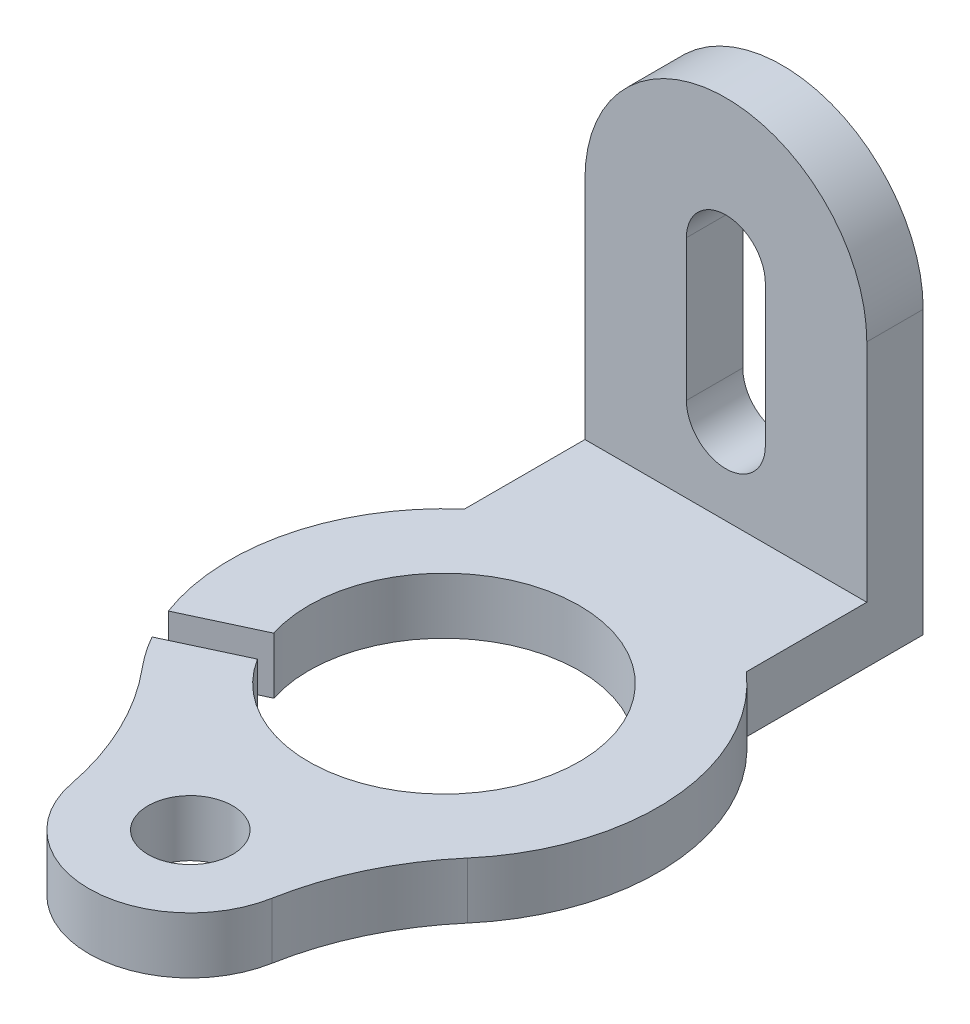
ISO-10303-21;
HEADER;
FILE_DESCRIPTION(('STEP AP214'),'2;1');
FILE_NAME('part.step','',(''),(''),'','','');
FILE_SCHEMA(('AUTOMOTIVE_DESIGN { 1 0 10303 214 1 1 1 1 }'));
ENDSEC;
DATA;
#1=APPLICATION_CONTEXT('core data for automotive mechanical design processes');
#2=APPLICATION_PROTOCOL_DEFINITION('international standard','automotive_design',2000,#1);
#3=PRODUCT_CONTEXT('',#1,'mechanical');
#4=PRODUCT('Part','Part','',(#3));
#5=PRODUCT_RELATED_PRODUCT_CATEGORY('part','',(#4));
#6=PRODUCT_DEFINITION_FORMATION('','',#4);
#7=PRODUCT_DEFINITION_CONTEXT('part definition',#1,'design');
#8=PRODUCT_DEFINITION('design','',#6,#7);
#9=PRODUCT_DEFINITION_SHAPE('','',#8);
#10=(LENGTH_UNIT() NAMED_UNIT(*) SI_UNIT(.MILLI.,.METRE.));
#11=(NAMED_UNIT(*) PLANE_ANGLE_UNIT() SI_UNIT($,.RADIAN.));
#12=(NAMED_UNIT(*) SI_UNIT($,.STERADIAN.) SOLID_ANGLE_UNIT());
#13=UNCERTAINTY_MEASURE_WITH_UNIT(LENGTH_MEASURE(1.E-05),#10,'distance_accuracy_value','');
#14=(GEOMETRIC_REPRESENTATION_CONTEXT(3) GLOBAL_UNCERTAINTY_ASSIGNED_CONTEXT((#13)) GLOBAL_UNIT_ASSIGNED_CONTEXT((#10,
#11,#12)) REPRESENTATION_CONTEXT('',''));
#15=CARTESIAN_POINT('',(0.,0.,0.));
#16=DIRECTION('',(0.,0.,1.));
#17=DIRECTION('',(1.,0.,0.));
#18=AXIS2_PLACEMENT_3D('',#15,#16,#17);
#19=CARTESIAN_POINT('',(-25.,5.,0.));
#20=DIRECTION('',(-1.,0.,0.));
#21=DIRECTION('',(0.,0.,1.));
#22=AXIS2_PLACEMENT_3D('',#19,#20,#21);
#23=PLANE('',#22);
#24=DIRECTION('',(0.,0.,-1.));
#25=VECTOR('',#24,1.);
#26=CARTESIAN_POINT('',(-25.,-5.,0.));
#27=LINE('',#26,#25);
#28=CARTESIAN_POINT('',(-25.,-5.,33.131068574005));
#29=VERTEX_POINT('',#28);
#30=CARTESIAN_POINT('',(-25.,-5.,1.74924461651332));
#31=VERTEX_POINT('',#30);
#32=EDGE_CURVE('E169',#29,#31,#27,.T.);
#33=ORIENTED_EDGE('',*,*,#32,.F.);
#34=DIRECTION('',(0.,-1.,0.));
#35=VECTOR('',#34,1.);
#36=CARTESIAN_POINT('',(-25.,5.,33.131068574005));
#37=LINE('',#36,#35);
#38=CARTESIAN_POINT('',(-25.,5.,33.131068574005));
#39=VERTEX_POINT('',#38);
#40=EDGE_CURVE('E11',#39,#29,#37,.T.);
#41=ORIENTED_EDGE('',*,*,#40,.F.);
#42=DIRECTION('',(0.,0.,-1.));
#43=VECTOR('',#42,1.);
#44=CARTESIAN_POINT('',(-25.,5.,0.));
#45=LINE('',#44,#43);
#46=CARTESIAN_POINT('',(-25.,5.,11.7492446165133));
#47=VERTEX_POINT('',#46);
#48=EDGE_CURVE('E232',#39,#47,#45,.T.);
#49=ORIENTED_EDGE('',*,*,#48,.T.);
#50=DIRECTION('',(0.,1.,0.));
#51=VECTOR('',#50,1.);
#52=CARTESIAN_POINT('',(-25.,-5.,11.7492446165133));
#53=LINE('',#52,#51);
#54=CARTESIAN_POINT('',(-25.,45.,11.7492446165133));
#55=VERTEX_POINT('',#54);
#56=EDGE_CURVE('E59',#47,#55,#53,.T.);
#57=ORIENTED_EDGE('',*,*,#56,.T.);
#58=DIRECTION('',(0.,0.,1.));
#59=VECTOR('',#58,1.);
#60=CARTESIAN_POINT('',(-25.,45.,1.74924461651332));
#61=LINE('',#60,#59);
#62=CARTESIAN_POINT('',(-25.,45.,1.74924461651332));
#63=VERTEX_POINT('',#62);
#64=EDGE_CURVE('E166',#63,#55,#61,.T.);
#65=ORIENTED_EDGE('',*,*,#64,.F.);
#66=DIRECTION('',(0.,1.,0.));
#67=VECTOR('',#66,1.);
#68=CARTESIAN_POINT('',(-25.,-5.,1.74924461651332));
#69=LINE('',#68,#67);
#70=EDGE_CURVE('E489',#31,#63,#69,.T.);
#71=ORIENTED_EDGE('',*,*,#70,.F.);
#72=EDGE_LOOP('',(#33,#41,#49,#57,#65,#71));
#73=FACE_BOUND('',#72,.T.);
#74=ADVANCED_FACE('F41',(#73),#23,.T.);
#75=CARTESIAN_POINT('',(0.,5.,61.7492446165134));
#76=DIRECTION('',(0.,-1.,0.));
#77=DIRECTION('',(0.,0.,-1.));
#78=AXIS2_PLACEMENT_3D('',#75,#76,#77);
#79=CYLINDRICAL_SURFACE('',#78,38.);
#80=CARTESIAN_POINT('',(0.,-5.,61.7492446165134));
#81=DIRECTION('',(0.,1.,0.));
#82=DIRECTION('',(0.,0.,1.));
#83=AXIS2_PLACEMENT_3D('',#80,#81,#82);
#84=CIRCLE('',#83,38.);
#85=CARTESIAN_POINT('',(-35.6000570150542,-5.,75.0396900765003));
#86=VERTEX_POINT('',#85);
#87=EDGE_CURVE('E171',#29,#86,#84,.T.);
#88=ORIENTED_EDGE('',*,*,#87,.T.);
#89=DIRECTION('',(0.,-1.,0.));
#90=VECTOR('',#89,1.);
#91=CARTESIAN_POINT('',(-35.6000570150542,5.,75.0396900765003));
#92=LINE('',#91,#90);
#93=CARTESIAN_POINT('',(-35.6000570150542,5.,75.0396900765003));
#94=VERTEX_POINT('',#93);
#95=EDGE_CURVE('E49',#94,#86,#92,.T.);
#96=ORIENTED_EDGE('',*,*,#95,.F.);
#97=CARTESIAN_POINT('',(0.,5.,61.7492446165134));
#98=DIRECTION('',(0.,1.,0.));
#99=DIRECTION('',(0.,0.,1.));
#100=AXIS2_PLACEMENT_3D('',#97,#98,#99);
#101=CIRCLE('',#100,38.);
#102=EDGE_CURVE('E227',#39,#94,#101,.T.);
#103=ORIENTED_EDGE('',*,*,#102,.F.);
#104=ORIENTED_EDGE('',*,*,#40,.T.);
#105=EDGE_LOOP('',(#88,#96,#103,#104));
#106=FACE_BOUND('',#105,.T.);
#107=ADVANCED_FACE('F218',(#106),#79,.T.);
#108=CARTESIAN_POINT('',(22.3834780674152,5.,48.0015236206457));
#109=DIRECTION('',(0.422618261740701,0.,0.906307787036649));
#110=DIRECTION('',(0.906307787036649,0.,-0.422618261740701));
#111=AXIS2_PLACEMENT_3D('',#108,#109,#110);
#112=PLANE('',#111);
#113=DIRECTION('',(-0.906307787036649,0.,0.422618261740701));
#114=VECTOR('',#113,1.);
#115=CARTESIAN_POINT('',(22.3834780674152,-5.,48.0015236206457));
#116=LINE('',#115,#114);
#117=CARTESIAN_POINT('',(-22.8486399272445,-5.,69.0936066361261));
#118=VERTEX_POINT('',#117);
#119=EDGE_CURVE('E172',#118,#86,#116,.T.);
#120=ORIENTED_EDGE('',*,*,#119,.F.);
#121=DIRECTION('',(0.,-1.,0.));
#122=VECTOR('',#121,1.);
#123=CARTESIAN_POINT('',(-22.8486399272445,5.,69.0936066361261));
#124=LINE('',#123,#122);
#125=CARTESIAN_POINT('',(-22.8486399272445,5.,69.0936066361261));
#126=VERTEX_POINT('',#125);
#127=EDGE_CURVE('E207',#126,#118,#124,.T.);
#128=ORIENTED_EDGE('',*,*,#127,.F.);
#129=DIRECTION('',(-0.906307787036649,0.,0.422618261740701));
#130=VECTOR('',#129,1.);
#131=CARTESIAN_POINT('',(22.3834780674152,5.,48.0015236206457));
#132=LINE('',#131,#130);
#133=EDGE_CURVE('E216',#126,#94,#132,.T.);
#134=ORIENTED_EDGE('',*,*,#133,.T.);
#135=ORIENTED_EDGE('',*,*,#95,.T.);
#136=EDGE_LOOP('',(#120,#128,#134,#135));
#137=FACE_BOUND('',#136,.T.);
#138=ADVANCED_FACE('F212',(#137),#112,.T.);
#139=CARTESIAN_POINT('',(0.,5.,61.7492446165134));
#140=DIRECTION('',(0.,-1.,0.));
#141=DIRECTION('',(0.,0.,-1.));
#142=AXIS2_PLACEMENT_3D('',#139,#140,#141);
#143=CYLINDRICAL_SURFACE('',#142,24.);
#144=CARTESIAN_POINT('',(0.,-5.,61.7492446165134));
#145=DIRECTION('',(0.,1.,0.));
#146=DIRECTION('',(0.,0.,1.));
#147=AXIS2_PLACEMENT_3D('',#144,#145,#146);
#148=CIRCLE('',#147,24.);
#149=CARTESIAN_POINT('',(-20.3129303568003,-5.,74.531453358346));
#150=VERTEX_POINT('',#149);
#151=EDGE_CURVE('E176',#150,#118,#148,.T.);
#152=ORIENTED_EDGE('',*,*,#151,.F.);
#153=DIRECTION('',(0.,-1.,0.));
#154=VECTOR('',#153,1.);
#155=CARTESIAN_POINT('',(-20.3129303568003,5.,74.531453358346));
#156=LINE('',#155,#154);
#157=CARTESIAN_POINT('',(-20.3129303568003,5.,74.531453358346));
#158=VERTEX_POINT('',#157);
#159=EDGE_CURVE('E210',#158,#150,#156,.T.);
#160=ORIENTED_EDGE('',*,*,#159,.F.);
#161=CARTESIAN_POINT('',(0.,5.,61.7492446165134));
#162=DIRECTION('',(0.,1.,0.));
#163=DIRECTION('',(0.,0.,1.));
#164=AXIS2_PLACEMENT_3D('',#161,#162,#163);
#165=CIRCLE('',#164,24.);
#166=EDGE_CURVE('E230',#158,#126,#165,.T.);
#167=ORIENTED_EDGE('',*,*,#166,.T.);
#168=ORIENTED_EDGE('',*,*,#127,.T.);
#169=EDGE_LOOP('',(#152,#160,#167,#168));
#170=FACE_BOUND('',#169,.T.);
#171=ADVANCED_FACE('F221',(#170),#143,.F.);
#172=CARTESIAN_POINT('',(24.9191876378595,5.,53.4393703428655));
#173=DIRECTION('',(0.422618261740702,0.,0.906307787036649));
#174=DIRECTION('',(0.906307787036649,0.,-0.422618261740702));
#175=AXIS2_PLACEMENT_3D('',#172,#173,#174);
#176=PLANE('',#175);
#177=DIRECTION('',(-0.906307787036649,0.,0.422618261740702));
#178=VECTOR('',#177,1.);
#179=CARTESIAN_POINT('',(24.9191876378595,-5.,53.4393703428655));
#180=LINE('',#179,#178);
#181=CARTESIAN_POINT('',(-33.06434744461,-5.,80.4775367987203));
#182=VERTEX_POINT('',#181);
#183=EDGE_CURVE('E182',#150,#182,#180,.T.);
#184=ORIENTED_EDGE('',*,*,#183,.T.);
#185=DIRECTION('',(0.,-1.,0.));
#186=VECTOR('',#185,1.);
#187=CARTESIAN_POINT('',(-33.06434744461,5.,80.4775367987203));
#188=LINE('',#187,#186);
#189=CARTESIAN_POINT('',(-33.06434744461,5.,80.4775367987203));
#190=VERTEX_POINT('',#189);
#191=EDGE_CURVE('E204',#190,#182,#188,.T.);
#192=ORIENTED_EDGE('',*,*,#191,.F.);
#193=DIRECTION('',(-0.906307787036649,0.,0.422618261740702));
#194=VECTOR('',#193,1.);
#195=CARTESIAN_POINT('',(24.9191876378595,5.,53.4393703428655));
#196=LINE('',#195,#194);
#197=EDGE_CURVE('E235',#158,#190,#196,.T.);
#198=ORIENTED_EDGE('',*,*,#197,.F.);
#199=ORIENTED_EDGE('',*,*,#159,.T.);
#200=EDGE_LOOP('',(#184,#192,#198,#199));
#201=FACE_BOUND('',#200,.T.);
#202=ADVANCED_FACE('F271',(#201),#176,.F.);
#203=CARTESIAN_POINT('',(0.,5.,61.7492446165134));
#204=DIRECTION('',(0.,-1.,0.));
#205=DIRECTION('',(0.,0.,-1.));
#206=AXIS2_PLACEMENT_3D('',#203,#204,#205);
#207=CYLINDRICAL_SURFACE('',#206,38.);
#208=CARTESIAN_POINT('',(0.,-5.,61.7492446165134));
#209=DIRECTION('',(0.,1.,0.));
#210=DIRECTION('',(0.,0.,1.));
#211=AXIS2_PLACEMENT_3D('',#208,#209,#210);
#212=CIRCLE('',#211,38.);
#213=CARTESIAN_POINT('',(-29.130311116903,-5.,86.1505760193783));
#214=VERTEX_POINT('',#213);
#215=EDGE_CURVE('E184',#182,#214,#212,.T.);
#216=ORIENTED_EDGE('',*,*,#215,.T.);
#217=DIRECTION('',(0.,-1.,0.));
#218=VECTOR('',#217,1.);
#219=CARTESIAN_POINT('',(-29.130311116903,5.,86.1505760193783));
#220=LINE('',#219,#218);
#221=CARTESIAN_POINT('',(-29.130311116903,5.,86.1505760193783));
#222=VERTEX_POINT('',#221);
#223=EDGE_CURVE('E205',#222,#214,#220,.T.);
#224=ORIENTED_EDGE('',*,*,#223,.F.);
#225=CARTESIAN_POINT('',(0.,5.,61.7492446165134));
#226=DIRECTION('',(0.,1.,0.));
#227=DIRECTION('',(0.,0.,1.));
#228=AXIS2_PLACEMENT_3D('',#225,#226,#227);
#229=CIRCLE('',#228,38.);
#230=EDGE_CURVE('E239',#190,#222,#229,.T.);
#231=ORIENTED_EDGE('',*,*,#230,.F.);
#232=ORIENTED_EDGE('',*,*,#191,.T.);
#233=EDGE_LOOP('',(#216,#224,#231,#232));
#234=FACE_BOUND('',#233,.T.);
#235=ADVANCED_FACE('F250',(#234),#207,.T.);
#236=CARTESIAN_POINT('',(-70.0123761004978,5.,120.395895682968));
#237=DIRECTION('',(0.,-1.,0.));
#238=DIRECTION('',(0.,0.,-1.));
#239=AXIS2_PLACEMENT_3D('',#236,#237,#238);
#240=CYLINDRICAL_SURFACE('',#239,53.3299648995226);
#241=CARTESIAN_POINT('',(-70.0123761004978,-5.,120.395895682968));
#242=DIRECTION('',(0.,1.,0.));
#243=DIRECTION('',(0.,0.,1.));
#244=AXIS2_PLACEMENT_3D('',#241,#242,#243);
#245=CIRCLE('',#244,53.3299648995226);
#246=CARTESIAN_POINT('',(-17.6675086211545,-5.,110.192954697434));
#247=VERTEX_POINT('',#246);
#248=EDGE_CURVE('E186',#247,#214,#245,.T.);
#249=ORIENTED_EDGE('',*,*,#248,.F.);
#250=DIRECTION('',(0.,-1.,0.));
#251=VECTOR('',#250,1.);
#252=CARTESIAN_POINT('',(-17.6675086211545,5.,110.192954697434));
#253=LINE('',#252,#251);
#254=CARTESIAN_POINT('',(-17.6675086211545,5.,110.192954697434));
#255=VERTEX_POINT('',#254);
#256=EDGE_CURVE('E199',#255,#247,#253,.T.);
#257=ORIENTED_EDGE('',*,*,#256,.F.);
#258=CARTESIAN_POINT('',(-70.0123761004978,5.,120.395895682968));
#259=DIRECTION('',(0.,1.,0.));
#260=DIRECTION('',(0.,0.,1.));
#261=AXIS2_PLACEMENT_3D('',#258,#259,#260);
#262=CIRCLE('',#261,53.3299648995226);
#263=EDGE_CURVE('E158',#255,#222,#262,.T.);
#264=ORIENTED_EDGE('',*,*,#263,.T.);
#265=ORIENTED_EDGE('',*,*,#223,.T.);
#266=EDGE_LOOP('',(#249,#257,#264,#265));
#267=FACE_BOUND('',#266,.T.);
#268=ADVANCED_FACE('F245',(#267),#240,.F.);
#269=CARTESIAN_POINT('',(0.,5.,106.749244616513));
#270=DIRECTION('',(0.,-1.,0.));
#271=DIRECTION('',(0.,0.,-1.));
#272=AXIS2_PLACEMENT_3D('',#269,#270,#271);
#273=CYLINDRICAL_SURFACE('',#272,18.);
#274=CARTESIAN_POINT('',(0.,-5.,106.749244616513));
#275=DIRECTION('',(0.,1.,0.));
#276=DIRECTION('',(0.,0.,1.));
#277=AXIS2_PLACEMENT_3D('',#274,#275,#276);
#278=CIRCLE('',#277,18.);
#279=CARTESIAN_POINT('',(17.711280988378,-5.,109.96024535627));
#280=VERTEX_POINT('',#279);
#281=EDGE_CURVE('E187',#247,#280,#278,.T.);
#282=ORIENTED_EDGE('',*,*,#281,.T.);
#283=DIRECTION('',(0.,-1.,0.));
#284=VECTOR('',#283,1.);
#285=CARTESIAN_POINT('',(17.711280988378,5.,109.96024535627));
#286=LINE('',#285,#284);
#287=CARTESIAN_POINT('',(17.711280988378,5.,109.96024535627));
#288=VERTEX_POINT('',#287);
#289=EDGE_CURVE('E139',#288,#280,#286,.T.);
#290=ORIENTED_EDGE('',*,*,#289,.F.);
#291=CARTESIAN_POINT('',(0.,5.,106.749244616513));
#292=DIRECTION('',(0.,1.,0.));
#293=DIRECTION('',(0.,0.,1.));
#294=AXIS2_PLACEMENT_3D('',#291,#292,#293);
#295=CIRCLE('',#294,18.);
#296=EDGE_CURVE('E154',#255,#288,#295,.T.);
#297=ORIENTED_EDGE('',*,*,#296,.F.);
#298=ORIENTED_EDGE('',*,*,#256,.T.);
#299=EDGE_LOOP('',(#282,#290,#297,#298));
#300=FACE_BOUND('',#299,.T.);
#301=ADVANCED_FACE('F249',(#300),#273,.T.);
#302=CARTESIAN_POINT('',(66.7753324792716,5.,118.855406905348));
#303=DIRECTION('',(0.,-1.,0.));
#304=DIRECTION('',(0.,0.,-1.));
#305=AXIS2_PLACEMENT_3D('',#302,#303,#304);
#306=CYLINDRICAL_SURFACE('',#305,49.8638651498784);
#307=CARTESIAN_POINT('',(66.7753324792716,-5.,118.855406905348));
#308=DIRECTION('',(0.,1.,0.));
#309=DIRECTION('',(0.,0.,1.));
#310=AXIS2_PLACEMENT_3D('',#307,#308,#309);
#311=CIRCLE('',#310,49.8638651498784);
#312=CARTESIAN_POINT('',(28.8794788379035,-5.,86.4469307844742));
#313=VERTEX_POINT('',#312);
#314=EDGE_CURVE('E137',#313,#280,#311,.T.);
#315=ORIENTED_EDGE('',*,*,#314,.F.);
#316=DIRECTION('',(0.,-1.,0.));
#317=VECTOR('',#316,1.);
#318=CARTESIAN_POINT('',(28.8794788379035,5.,86.4469307844742));
#319=LINE('',#318,#317);
#320=CARTESIAN_POINT('',(28.8794788379035,5.,86.4469307844742));
#321=VERTEX_POINT('',#320);
#322=EDGE_CURVE('E94',#321,#313,#319,.T.);
#323=ORIENTED_EDGE('',*,*,#322,.F.);
#324=CARTESIAN_POINT('',(66.7753324792716,5.,118.855406905348));
#325=DIRECTION('',(0.,1.,0.));
#326=DIRECTION('',(0.,0.,1.));
#327=AXIS2_PLACEMENT_3D('',#324,#325,#326);
#328=CIRCLE('',#327,49.8638651498784);
#329=EDGE_CURVE('E140',#321,#288,#328,.T.);
#330=ORIENTED_EDGE('',*,*,#329,.T.);
#331=ORIENTED_EDGE('',*,*,#289,.T.);
#332=EDGE_LOOP('',(#315,#323,#330,#331));
#333=FACE_BOUND('',#332,.T.);
#334=ADVANCED_FACE('F132',(#333),#306,.F.);
#335=CARTESIAN_POINT('',(0.,5.,61.7492446165134));
#336=DIRECTION('',(0.,-1.,0.));
#337=DIRECTION('',(0.,0.,-1.));
#338=AXIS2_PLACEMENT_3D('',#335,#336,#337);
#339=CYLINDRICAL_SURFACE('',#338,38.);
#340=CARTESIAN_POINT('',(0.,-5.,61.7492446165134));
#341=DIRECTION('',(0.,1.,0.));
#342=DIRECTION('',(0.,0.,1.));
#343=AXIS2_PLACEMENT_3D('',#340,#341,#342);
#344=CIRCLE('',#343,38.);
#345=CARTESIAN_POINT('',(25.,-5.,33.1310685740051));
#346=VERTEX_POINT('',#345);
#347=EDGE_CURVE('E192',#313,#346,#344,.T.);
#348=ORIENTED_EDGE('',*,*,#347,.T.);
#349=DIRECTION('',(0.,-1.,0.));
#350=VECTOR('',#349,1.);
#351=CARTESIAN_POINT('',(25.,5.,33.1310685740051));
#352=LINE('',#351,#350);
#353=CARTESIAN_POINT('',(25.,5.,33.1310685740051));
#354=VERTEX_POINT('',#353);
#355=EDGE_CURVE('E143',#354,#346,#352,.T.);
#356=ORIENTED_EDGE('',*,*,#355,.F.);
#357=CARTESIAN_POINT('',(0.,5.,61.7492446165134));
#358=DIRECTION('',(0.,1.,0.));
#359=DIRECTION('',(0.,0.,1.));
#360=AXIS2_PLACEMENT_3D('',#357,#358,#359);
#361=CIRCLE('',#360,38.);
#362=EDGE_CURVE('E144',#321,#354,#361,.T.);
#363=ORIENTED_EDGE('',*,*,#362,.F.);
#364=ORIENTED_EDGE('',*,*,#322,.T.);
#365=EDGE_LOOP('',(#348,#356,#363,#364));
#366=FACE_BOUND('',#365,.T.);
#367=ADVANCED_FACE('F148',(#366),#339,.T.);
#368=CARTESIAN_POINT('',(25.,5.,0.));
#369=DIRECTION('',(-1.,0.,0.));
#370=DIRECTION('',(0.,0.,1.));
#371=AXIS2_PLACEMENT_3D('',#368,#369,#370);
#372=PLANE('',#371);
#373=DIRECTION('',(0.,0.,-1.));
#374=VECTOR('',#373,1.);
#375=CARTESIAN_POINT('',(25.,-5.,0.));
#376=LINE('',#375,#374);
#377=CARTESIAN_POINT('',(25.,-5.,1.74924461651332));
#378=VERTEX_POINT('',#377);
#379=EDGE_CURVE('E101',#346,#378,#376,.T.);
#380=ORIENTED_EDGE('',*,*,#379,.T.);
#381=DIRECTION('',(0.,-1.,0.));
#382=VECTOR('',#381,1.);
#383=CARTESIAN_POINT('',(25.,-5.,1.74924461651332));
#384=LINE('',#383,#382);
#385=CARTESIAN_POINT('',(25.,45.,1.74924461651332));
#386=VERTEX_POINT('',#385);
#387=EDGE_CURVE('E500',#386,#378,#384,.T.);
#388=ORIENTED_EDGE('',*,*,#387,.F.);
#389=DIRECTION('',(0.,0.,1.));
#390=VECTOR('',#389,1.);
#391=CARTESIAN_POINT('',(25.,45.,1.74924461651332));
#392=LINE('',#391,#390);
#393=CARTESIAN_POINT('',(25.,45.,11.7492446165133));
#394=VERTEX_POINT('',#393);
#395=EDGE_CURVE('E498',#386,#394,#392,.T.);
#396=ORIENTED_EDGE('',*,*,#395,.T.);
#397=DIRECTION('',(0.,-1.,0.));
#398=VECTOR('',#397,1.);
#399=CARTESIAN_POINT('',(25.,-5.,11.7492446165133));
#400=LINE('',#399,#398);
#401=CARTESIAN_POINT('',(25.,5.,11.7492446165133));
#402=VERTEX_POINT('',#401);
#403=EDGE_CURVE('E491',#394,#402,#400,.T.);
#404=ORIENTED_EDGE('',*,*,#403,.T.);
#405=DIRECTION('',(0.,0.,-1.));
#406=VECTOR('',#405,1.);
#407=CARTESIAN_POINT('',(25.,5.,0.));
#408=LINE('',#407,#406);
#409=EDGE_CURVE('E149',#354,#402,#408,.T.);
#410=ORIENTED_EDGE('',*,*,#409,.F.);
#411=ORIENTED_EDGE('',*,*,#355,.T.);
#412=EDGE_LOOP('',(#380,#388,#396,#404,#410,#411));
#413=FACE_BOUND('',#412,.T.);
#414=ADVANCED_FACE('F304',(#413),#372,.F.);
#415=CARTESIAN_POINT('',(0.,5.,106.749244616513));
#416=DIRECTION('',(0.,-1.,0.));
#417=DIRECTION('',(0.,0.,-1.));
#418=AXIS2_PLACEMENT_3D('',#415,#416,#417);
#419=CYLINDRICAL_SURFACE('',#418,7.50000000000001);
#420=CARTESIAN_POINT('',(0.,5.,106.749244616513));
#421=DIRECTION('',(0.,1.,0.));
#422=DIRECTION('',(0.,0.,1.));
#423=AXIS2_PLACEMENT_3D('',#420,#421,#422);
#424=CIRCLE('',#423,7.50000000000001);
#425=CARTESIAN_POINT('',(0.,5.,114.249244616513));
#426=VERTEX_POINT('',#425);
#427=EDGE_CURVE('E197',#426,#426,#424,.T.);
#428=ORIENTED_EDGE('',*,*,#427,.T.);
#429=EDGE_LOOP('',(#428));
#430=FACE_BOUND('',#429,.T.);
#431=CARTESIAN_POINT('',(0.,-5.,106.749244616513));
#432=DIRECTION('',(0.,1.,0.));
#433=DIRECTION('',(0.,0.,1.));
#434=AXIS2_PLACEMENT_3D('',#431,#432,#433);
#435=CIRCLE('',#434,7.50000000000001);
#436=CARTESIAN_POINT('',(0.,-5.,114.249244616513));
#437=VERTEX_POINT('',#436);
#438=EDGE_CURVE('E164',#437,#437,#435,.T.);
#439=ORIENTED_EDGE('',*,*,#438,.F.);
#440=EDGE_LOOP('',(#439));
#441=FACE_BOUND('',#440,.T.);
#442=ADVANCED_FACE('F43',(#430,#441),#419,.F.);
#443=CARTESIAN_POINT('',(0.,5.,0.));
#444=DIRECTION('',(0.,1.,0.));
#445=DIRECTION('',(0.,0.,1.));
#446=AXIS2_PLACEMENT_3D('',#443,#444,#445);
#447=PLANE('',#446);
#448=ORIENTED_EDGE('',*,*,#427,.F.);
#449=EDGE_LOOP('',(#448));
#450=FACE_BOUND('',#449,.T.);
#451=ORIENTED_EDGE('',*,*,#48,.F.);
#452=ORIENTED_EDGE('',*,*,#102,.T.);
#453=ORIENTED_EDGE('',*,*,#133,.F.);
#454=ORIENTED_EDGE('',*,*,#166,.F.);
#455=ORIENTED_EDGE('',*,*,#197,.T.);
#456=ORIENTED_EDGE('',*,*,#230,.T.);
#457=ORIENTED_EDGE('',*,*,#263,.F.);
#458=ORIENTED_EDGE('',*,*,#296,.T.);
#459=ORIENTED_EDGE('',*,*,#329,.F.);
#460=ORIENTED_EDGE('',*,*,#362,.T.);
#461=ORIENTED_EDGE('',*,*,#409,.T.);
#462=DIRECTION('',(-1.,0.,0.));
#463=VECTOR('',#462,1.);
#464=CARTESIAN_POINT('',(0.,5.,11.7492446165133));
#465=LINE('',#464,#463);
#466=EDGE_CURVE('E162',#402,#47,#465,.T.);
#467=ORIENTED_EDGE('',*,*,#466,.T.);
#468=EDGE_LOOP('',(#451,#452,#453,#454,#455,#456,#457,#458,#459,#460,#461,#467));
#469=FACE_BOUND('',#468,.T.);
#470=ADVANCED_FACE('F155',(#450,#469),#447,.T.);
#471=CARTESIAN_POINT('',(0.,-5.,0.));
#472=DIRECTION('',(0.,1.,0.));
#473=DIRECTION('',(0.,0.,1.));
#474=AXIS2_PLACEMENT_3D('',#471,#472,#473);
#475=PLANE('',#474);
#476=ORIENTED_EDGE('',*,*,#438,.T.);
#477=EDGE_LOOP('',(#476));
#478=FACE_BOUND('',#477,.T.);
#479=ORIENTED_EDGE('',*,*,#32,.T.);
#480=DIRECTION('',(-1.,0.,0.));
#481=VECTOR('',#480,1.);
#482=CARTESIAN_POINT('',(25.,-5.,1.74924461651332));
#483=LINE('',#482,#481);
#484=EDGE_CURVE('E490',#378,#31,#483,.T.);
#485=ORIENTED_EDGE('',*,*,#484,.F.);
#486=ORIENTED_EDGE('',*,*,#379,.F.);
#487=ORIENTED_EDGE('',*,*,#347,.F.);
#488=ORIENTED_EDGE('',*,*,#314,.T.);
#489=ORIENTED_EDGE('',*,*,#281,.F.);
#490=ORIENTED_EDGE('',*,*,#248,.T.);
#491=ORIENTED_EDGE('',*,*,#215,.F.);
#492=ORIENTED_EDGE('',*,*,#183,.F.);
#493=ORIENTED_EDGE('',*,*,#151,.T.);
#494=ORIENTED_EDGE('',*,*,#119,.T.);
#495=ORIENTED_EDGE('',*,*,#87,.F.);
#496=EDGE_LOOP('',(#479,#485,#486,#487,#488,#489,#490,#491,#492,#493,#494,#495));
#497=FACE_BOUND('',#496,.T.);
#498=ADVANCED_FACE('F219',(#478,#497),#475,.F.);
#499=CARTESIAN_POINT('',(0.,45.,1.74924461651332));
#500=DIRECTION('',(0.,0.,-1.));
#501=DIRECTION('',(-1.,0.,0.));
#502=AXIS2_PLACEMENT_3D('',#499,#500,#501);
#503=PLANE('',#502);
#504=ORIENTED_EDGE('',*,*,#484,.T.);
#505=ORIENTED_EDGE('',*,*,#70,.T.);
#506=CARTESIAN_POINT('',(0.,45.,1.74924461651332));
#507=DIRECTION('',(0.,0.,-1.));
#508=DIRECTION('',(-1.,0.,0.));
#509=AXIS2_PLACEMENT_3D('',#506,#507,#508);
#510=CIRCLE('',#509,25.);
#511=EDGE_CURVE('E493',#63,#386,#510,.T.);
#512=ORIENTED_EDGE('',*,*,#511,.T.);
#513=ORIENTED_EDGE('',*,*,#387,.T.);
#514=EDGE_LOOP('',(#504,#505,#512,#513));
#515=FACE_BOUND('',#514,.T.);
#516=DIRECTION('',(0.,-1.,0.));
#517=VECTOR('',#516,1.);
#518=CARTESIAN_POINT('',(7.,45.,1.74924461651332));
#519=LINE('',#518,#517);
#520=CARTESIAN_POINT('',(7.,45.,1.74924461651332));
#521=VERTEX_POINT('',#520);
#522=CARTESIAN_POINT('',(7.,20.,1.74924461651332));
#523=VERTEX_POINT('',#522);
#524=EDGE_CURVE('E539',#521,#523,#519,.T.);
#525=ORIENTED_EDGE('',*,*,#524,.F.);
#526=CARTESIAN_POINT('',(0.,45.,1.74924461651332));
#527=DIRECTION('',(0.,0.,-1.));
#528=DIRECTION('',(-1.,0.,0.));
#529=AXIS2_PLACEMENT_3D('',#526,#527,#528);
#530=CIRCLE('',#529,7.);
#531=CARTESIAN_POINT('',(-7.,45.,1.74924461651332));
#532=VERTEX_POINT('',#531);
#533=EDGE_CURVE('E462',#532,#521,#530,.T.);
#534=ORIENTED_EDGE('',*,*,#533,.F.);
#535=DIRECTION('',(0.,1.,0.));
#536=VECTOR('',#535,1.);
#537=CARTESIAN_POINT('',(-7.,45.,1.74924461651332));
#538=LINE('',#537,#536);
#539=CARTESIAN_POINT('',(-7.,20.,1.74924461651332));
#540=VERTEX_POINT('',#539);
#541=EDGE_CURVE('E479',#540,#532,#538,.T.);
#542=ORIENTED_EDGE('',*,*,#541,.F.);
#543=CARTESIAN_POINT('',(0.,20.,1.74924461651332));
#544=DIRECTION('',(0.,0.,-1.));
#545=DIRECTION('',(-1.,0.,0.));
#546=AXIS2_PLACEMENT_3D('',#543,#544,#545);
#547=CIRCLE('',#546,7.);
#548=EDGE_CURVE('E538',#523,#540,#547,.T.);
#549=ORIENTED_EDGE('',*,*,#548,.F.);
#550=EDGE_LOOP('',(#525,#534,#542,#549));
#551=FACE_BOUND('',#550,.T.);
#552=ADVANCED_FACE('F337',(#515,#551),#503,.T.);
#553=CARTESIAN_POINT('',(0.,45.,11.7492446165133));
#554=DIRECTION('',(0.,0.,-1.));
#555=DIRECTION('',(-1.,0.,0.));
#556=AXIS2_PLACEMENT_3D('',#553,#554,#555);
#557=PLANE('',#556);
#558=ORIENTED_EDGE('',*,*,#466,.F.);
#559=ORIENTED_EDGE('',*,*,#403,.F.);
#560=CARTESIAN_POINT('',(0.,45.,11.7492446165133));
#561=DIRECTION('',(0.,0.,-1.));
#562=DIRECTION('',(-1.,0.,0.));
#563=AXIS2_PLACEMENT_3D('',#560,#561,#562);
#564=CIRCLE('',#563,25.);
#565=EDGE_CURVE('E501',#55,#394,#564,.T.);
#566=ORIENTED_EDGE('',*,*,#565,.F.);
#567=ORIENTED_EDGE('',*,*,#56,.F.);
#568=EDGE_LOOP('',(#558,#559,#566,#567));
#569=FACE_BOUND('',#568,.T.);
#570=CARTESIAN_POINT('',(0.,45.,11.7492446165133));
#571=DIRECTION('',(0.,0.,-1.));
#572=DIRECTION('',(-1.,0.,0.));
#573=AXIS2_PLACEMENT_3D('',#570,#571,#572);
#574=CIRCLE('',#573,7.);
#575=CARTESIAN_POINT('',(-7.,45.,11.7492446165133));
#576=VERTEX_POINT('',#575);
#577=CARTESIAN_POINT('',(7.,45.,11.7492446165133));
#578=VERTEX_POINT('',#577);
#579=EDGE_CURVE('E475',#576,#578,#574,.T.);
#580=ORIENTED_EDGE('',*,*,#579,.T.);
#581=DIRECTION('',(0.,-1.,0.));
#582=VECTOR('',#581,1.);
#583=CARTESIAN_POINT('',(7.,45.,11.7492446165133));
#584=LINE('',#583,#582);
#585=CARTESIAN_POINT('',(7.,20.,11.7492446165133));
#586=VERTEX_POINT('',#585);
#587=EDGE_CURVE('E473',#578,#586,#584,.T.);
#588=ORIENTED_EDGE('',*,*,#587,.T.);
#589=CARTESIAN_POINT('',(0.,20.,11.7492446165133));
#590=DIRECTION('',(0.,0.,-1.));
#591=DIRECTION('',(-1.,0.,0.));
#592=AXIS2_PLACEMENT_3D('',#589,#590,#591);
#593=CIRCLE('',#592,7.);
#594=CARTESIAN_POINT('',(-7.,20.,11.7492446165133));
#595=VERTEX_POINT('',#594);
#596=EDGE_CURVE('E468',#586,#595,#593,.T.);
#597=ORIENTED_EDGE('',*,*,#596,.T.);
#598=DIRECTION('',(0.,1.,0.));
#599=VECTOR('',#598,1.);
#600=CARTESIAN_POINT('',(-7.,45.,11.7492446165133));
#601=LINE('',#600,#599);
#602=EDGE_CURVE('E447',#595,#576,#601,.T.);
#603=ORIENTED_EDGE('',*,*,#602,.T.);
#604=EDGE_LOOP('',(#580,#588,#597,#603));
#605=FACE_BOUND('',#604,.T.);
#606=ADVANCED_FACE('F382',(#569,#605),#557,.F.);
#607=CARTESIAN_POINT('',(0.,45.,1.74924461651332));
#608=DIRECTION('',(0.,0.,1.));
#609=DIRECTION('',(1.,0.,0.));
#610=AXIS2_PLACEMENT_3D('',#607,#608,#609);
#611=CYLINDRICAL_SURFACE('',#610,25.);
#612=ORIENTED_EDGE('',*,*,#565,.T.);
#613=ORIENTED_EDGE('',*,*,#395,.F.);
#614=ORIENTED_EDGE('',*,*,#511,.F.);
#615=ORIENTED_EDGE('',*,*,#64,.T.);
#616=EDGE_LOOP('',(#612,#613,#614,#615));
#617=FACE_BOUND('',#616,.T.);
#618=ADVANCED_FACE('F395',(#617),#611,.T.);
#619=CARTESIAN_POINT('',(0.,45.,1.74924461651332));
#620=DIRECTION('',(0.,0.,1.));
#621=DIRECTION('',(1.,0.,0.));
#622=AXIS2_PLACEMENT_3D('',#619,#620,#621);
#623=CYLINDRICAL_SURFACE('',#622,7.);
#624=ORIENTED_EDGE('',*,*,#579,.F.);
#625=DIRECTION('',(0.,0.,1.));
#626=VECTOR('',#625,1.);
#627=CARTESIAN_POINT('',(-7.,45.,1.74924461651332));
#628=LINE('',#627,#626);
#629=EDGE_CURVE('E459',#532,#576,#628,.T.);
#630=ORIENTED_EDGE('',*,*,#629,.F.);
#631=ORIENTED_EDGE('',*,*,#533,.T.);
#632=DIRECTION('',(0.,0.,1.));
#633=VECTOR('',#632,1.);
#634=CARTESIAN_POINT('',(7.,45.,1.74924461651332));
#635=LINE('',#634,#633);
#636=EDGE_CURVE('E482',#521,#578,#635,.T.);
#637=ORIENTED_EDGE('',*,*,#636,.T.);
#638=EDGE_LOOP('',(#624,#630,#631,#637));
#639=FACE_BOUND('',#638,.T.);
#640=ADVANCED_FACE('F405',(#639),#623,.F.);
#641=CARTESIAN_POINT('',(7.,45.,1.74924461651332));
#642=DIRECTION('',(-1.,0.,0.));
#643=DIRECTION('',(0.,-1.,0.));
#644=AXIS2_PLACEMENT_3D('',#641,#642,#643);
#645=PLANE('',#644);
#646=ORIENTED_EDGE('',*,*,#587,.F.);
#647=ORIENTED_EDGE('',*,*,#636,.F.);
#648=ORIENTED_EDGE('',*,*,#524,.T.);
#649=DIRECTION('',(0.,0.,1.));
#650=VECTOR('',#649,1.);
#651=CARTESIAN_POINT('',(7.,20.,1.74924461651332));
#652=LINE('',#651,#650);
#653=EDGE_CURVE('E481',#523,#586,#652,.T.);
#654=ORIENTED_EDGE('',*,*,#653,.T.);
#655=EDGE_LOOP('',(#646,#647,#648,#654));
#656=FACE_BOUND('',#655,.T.);
#657=ADVANCED_FACE('F415',(#656),#645,.T.);
#658=CARTESIAN_POINT('',(0.,20.,1.74924461651332));
#659=DIRECTION('',(0.,0.,1.));
#660=DIRECTION('',(1.,0.,0.));
#661=AXIS2_PLACEMENT_3D('',#658,#659,#660);
#662=CYLINDRICAL_SURFACE('',#661,7.);
#663=ORIENTED_EDGE('',*,*,#596,.F.);
#664=ORIENTED_EDGE('',*,*,#653,.F.);
#665=ORIENTED_EDGE('',*,*,#548,.T.);
#666=DIRECTION('',(0.,0.,1.));
#667=VECTOR('',#666,1.);
#668=CARTESIAN_POINT('',(-7.,20.,1.74924461651332));
#669=LINE('',#668,#667);
#670=EDGE_CURVE('E454',#540,#595,#669,.T.);
#671=ORIENTED_EDGE('',*,*,#670,.T.);
#672=EDGE_LOOP('',(#663,#664,#665,#671));
#673=FACE_BOUND('',#672,.T.);
#674=ADVANCED_FACE('F425',(#673),#662,.F.);
#675=CARTESIAN_POINT('',(-7.,45.,1.74924461651332));
#676=DIRECTION('',(1.,0.,0.));
#677=DIRECTION('',(0.,1.,0.));
#678=AXIS2_PLACEMENT_3D('',#675,#676,#677);
#679=PLANE('',#678);
#680=ORIENTED_EDGE('',*,*,#602,.F.);
#681=ORIENTED_EDGE('',*,*,#670,.F.);
#682=ORIENTED_EDGE('',*,*,#541,.T.);
#683=ORIENTED_EDGE('',*,*,#629,.T.);
#684=EDGE_LOOP('',(#680,#681,#682,#683));
#685=FACE_BOUND('',#684,.T.);
#686=ADVANCED_FACE('F435',(#685),#679,.T.);
#687=CLOSED_SHELL('',(#74,#107,#138,#171,#202,#235,#268,#301,#334,#367,#414,#442,#470,#498,#552,
#606,#618,#640,#657,#674,#686));
#688=MANIFOLD_SOLID_BREP('B2',#687);
#689=ADVANCED_BREP_SHAPE_REPRESENTATION('',(#18,#688),#14);
#690=SHAPE_DEFINITION_REPRESENTATION(#9,#689);
ENDSEC;
END-ISO-10303-21;
